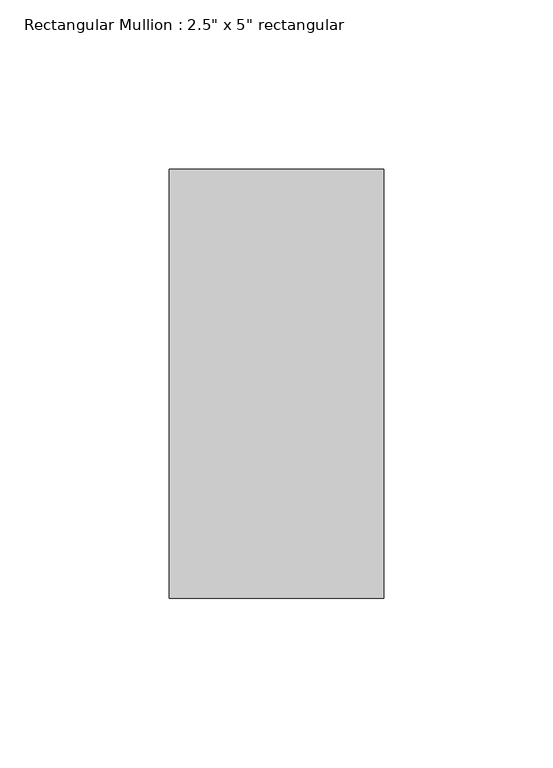
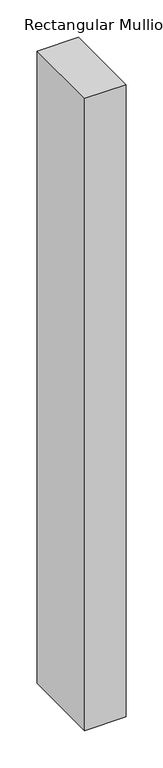
"""IFC4 building model written with IfcOpenShell, lengths in millimetres: member geometry."""

from ifc_helpers import new_model, si_unit, frame, origin, place, context, project, spatial, polyline, outline, extrude, source, transform, mapped, element, save


def member_20160837(model_context):
    return source(origin(), model_context, "Body", "SweptSolid", [
        extrude(outline(polyline([(31.75, 63.5), (31.75, -63.5), (-31.75, -63.5), (-31.75, 63.5), (31.75, 63.5)])), frame((0.0, 0.0, -1031.7272807), z_axis=(0.0, 0.0, 1.0), x_axis=(1.0, 0.0, 0.0)), (0.0, 0.0, 1.0), 1031.7272807),
    ])


if __name__ == "__main__":
    model = new_model("IFC4")
    model_context = context("Model", 3, world=origin())
    ifc_project = project(units=[si_unit("LENGTHUNIT", "METRE", prefix="MILLI")], contexts=[model_context])
    site = spatial("IfcSite", under=ifc_project)
    building = spatial("IfcBuilding", under=site)
    placement = place(None, origin())
    member_shape = member_20160837(model_context)
    element("IfcMember", 1, ObjectType="Rectangular Mullion : 2.5\" x 5\" rectangular", at=placement, inside=building, context=model_context, shape_type="MappedRepresentation", body=[
        mapped(member_shape, transform((0.0, 0.0, 0.0), x_axis=(1.0, 0.0, 0.0), y_axis=(0.0, 1.0, 0.0), z_axis=(0.0, 0.0, 1.0))),
    ])
    save(model, "model.ifc")

# Revit data of these elements
# Type "Rectangular Mullion : 2.5\" x 5\" rectangular"
#   built-in parameter 1007304 = 0.416667 (stored number, unit not read)
#   built-in parameter 1007301 = 0.104167 (stored number, unit not read)
#   built-in parameter 1007300 = 0.104167 (stored number, unit not read)
# Element 1 (IfcMember, "Rectangular Mullion : 2.5\" x 5\" rectangular")
#   Materials on its faces: "Aluminum"
# Materials
#   "Aluminum": class "Metal", colour RGB 247 247 247, transparency 0, Description = "Aluminum 6061", Cost = 0
